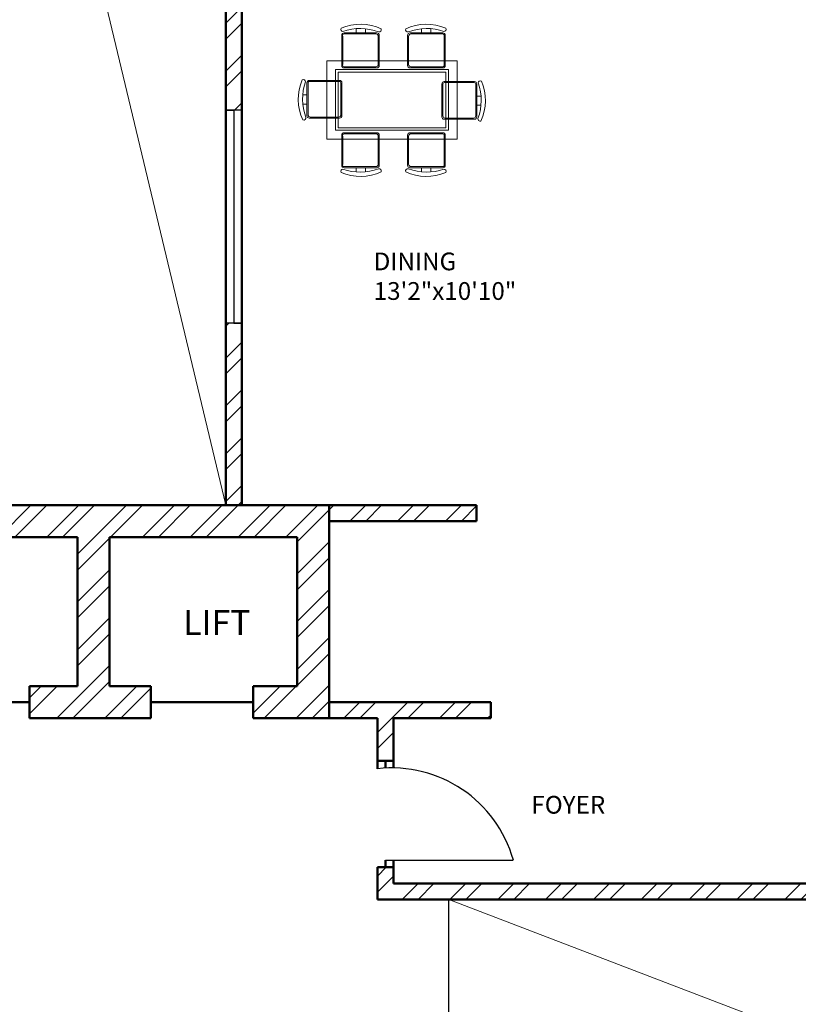
# Model space of a CAD drawing. Units: inches. Extents: x 1901 to 2863, y 888 to 2433.
# Tile 66 of 91: x 2381 to 2601, y 1732 to 2009. Entities that reach past the tile are written whole.
import ezdxf

# ---------------------------------------------------------------- set-up
doc = ezdxf.new("R2010")
doc.units = ezdxf.units.IN
for name, color, linetype, lineweight in [('A-ANNO-SYMB', 8, 'Continuous', 13), ('A-AREA-IDEN', 7, 'Continuous', 18), ('A-DOOR', 4, 'Continuous', 25), ('A-FLOR-HRAL', 41, 'Continuous', 25), ('A-FURN', 8, 'Continuous', 18), ('A-GLAZ', 3, 'Continuous', 25), ('A-WALL', 7, 'Continuous', 50), ('A-WALL-PATT', 8, 'Continuous', 13)]:
    doc.layers.add(name, color=color, linetype=linetype, lineweight=lineweight)
doc.styles.get("Standard").update_dxf_attribs({"font": 'arial.ttf'})

# ---------------------------------------------------------------- blocks, each defined once
blk = doc.blocks.new('WIN-60')
for p, q in [((0, 4.5), (0, 0)), ((60, 2.25), (60, 4.5)), ((60, 4.5), (60, 0)), ((0, 0), (0, 2.25)), ((0, 2.25), (60, 2.25))]:
    blk.add_line(p, q)

msp = doc.modelspace()

# ---------------------------------------------------------------- hatches: boundary and pattern name
at = {"layer": 'A-WALL-PATT'}
h = msp.add_hatch(dxfattribs=at)
h.set_pattern_fill('ANSI32', color=256)
h.paths.add_polyline_path([(2192.5, 2274.13), (2141.26, 2274.13), (2141.26, 2269.63), (2192.5, 2269.63)])
h.paths.add_polyline_path([(2259.93, 2274.13), (2216.5, 2274.13), (2216.5, 2269.63), (2255.43, 2269.63), (2255.43, 2214.63), (2250.81, 2214.63), (2250.81, 2210.13), (2259.93, 2210.13), (2259.93, 2215.13), (2271.76, 2215.13), (2271.76, 2217.38), (2271.76, 2219.63), (2259.93, 2219.63)])
h.paths.add_polyline_path([(2171.43, 2269.63), (2166.93, 2269.63), (2166.93, 2219.63), (2121.24, 2219.63), (2121.24, 2215.13), (2166.93, 2215.13), (2166.93, 2083.13), (2161.81, 2083.13), (2161.81, 2078.63), (2171.43, 2078.63), (2177, 2078.63), (2177, 2080.88), (2177, 2083.13), (2171.43, 2083.13), (2171.43, 2210.13), (2230.91, 2210.13), (2230.91, 2212.38), (2230.91, 2214.63), (2171.43, 2214.63)])
h.paths.add_polyline_path([(2117.26, 2274.13), (2089.43, 2274.13), (2089.43, 2219.63), (2081.14, 2219.63), (2081.14, 2215.13), (2089.43, 2215.13), (2098, 2215.13), (2098, 2217.38), (2098, 2219.63), (2093.93, 2219.63), (2093.93, 2269.63), (2117.26, 2269.63), (2117.26, 2271.88)])
h.paths.add_polyline_path([(2343.43, 2219.63), (2329.29, 2219.63), (2329.29, 2215.13), (2338.93, 2215.13), (2338.93, 2184.74), (2343.43, 2184.74)])
h.paths.add_polyline_path([(2338.93, 2083.13), (2329.29, 2083.13), (2208.97, 2083.13), (2208.97, 2078.63), (2338.93, 2078.63)])
h.paths.add_polyline_path([(2343.43, 2136.74), (2338.93, 2136.74), (2338.93, 1872.63), (2343.43, 1872.63)])
h.paths.add_polyline_path([(2343.43, 1863.63), (2397.68, 1863.63), (2397.68, 1821.63), (2384.14, 1821.63), (2384.14, 1812.63), (2418.33, 1812.63), (2418.33, 1817.13), (2418.33, 1821.63), (2406.68, 1821.63), (2406.68, 1863.63), (2459.5, 1863.63), (2459.5, 1821.63), (2447.14, 1821.63), (2447.14, 1812.63), (2459.5, 1812.63), (2468.5, 1812.63), (2468.5, 1872.63), (2394.43, 1872.63), (2334.43, 1872.63), (2334.43, 1812.63), (2343.43, 1812.63), (2353.25, 1812.63), (2353.25, 1821.63), (2343.43, 1821.63)])
h.paths.add_polyline_path([(2510.01, 1872.63), (2468.5, 1872.63), (2468.5, 1868.13), (2510.01, 1868.13)])
h.paths.add_polyline_path([(2514.01, 1817.13), (2468.5, 1817.13), (2468.5, 1812.63), (2482.11, 1812.63), (2482.11, 1800.61), (2486.61, 1800.61), (2486.61, 1812.63), (2514.01, 1812.63)])
h.paths.add_polyline_path([(2299.25, 1814.88), (2299.25, 1817.13), (2295.93, 1817.13), (2295.93, 1854.17), (2293.68, 1854.17), (2291.43, 1854.17), (2291.43, 1817.13), (2266.11, 1817.13), (2266.11, 1812.63), (2299.25, 1812.63)])
h.paths.add_polyline_path([(2218.11, 1817.13), (2206.46, 1817.13), (2171.43, 1817.13), (2171.43, 1949.13), (2190.1, 1949.13), (2190.1, 1953.63), (2163.47, 1953.63), (2163.47, 1949.13), (2166.93, 1949.13), (2166.93, 1817.13), (2114.3, 1817.13), (2114.3, 1812.63), (2218.11, 1812.63)])
h.paths.add_polyline_path([(2029.43, 1970.92), (2024.93, 1970.92), (2024.93, 1912.72), (2029.43, 1912.72)])
h.paths.add_polyline_path([(2132.3, 1953.63), (2113.93, 1953.63), (2113.93, 1975.89), (2111.68, 1975.89), (2109.43, 1975.89), (2109.43, 1953.63), (2029.43, 1953.63), (2029.43, 1949.13), (2132.3, 1949.13)])
h.paths.add_polyline_path([(2029.43, 1853.61), (2029.31, 1853.61), (2029.31, 1853.61), (2029.43, 1853.61), (2029.43, 1864.72), (2024.93, 1864.72), (2024.93, 1812.63), (2066.3, 1812.63), (2066.3, 1814.88), (2066.3, 1817.13), (2029.43, 1817.13)])
h.paths.add_polyline_path([(2122.93, 2010.09), (2120.68, 2010.09), (2118.43, 2010.09), (2118.43, 2006.13), (2029.43, 2006.13), (2029.43, 2001.63), (2109.43, 2001.63), (2109.43, 1998.04), (2113.93, 1998.04), (2113.93, 2001.63), (2122.93, 2001.63)])
h.paths.add_polyline_path([(2029.43, 2031.38), (2024.93, 2031.38), (2024.93, 1994.92), (2027.18, 1994.92), (2029.43, 1994.92)])
h.paths.add_polyline_path([(2029.43, 2136.74), (2024.93, 2136.74), (2024.93, 2067.38), (2027.18, 2067.38), (2029.43, 2067.38)])
h.paths.add_polyline_path([(2125.62, 2083.13), (2029.43, 2083.13), (2029.43, 2078.63), (2118.43, 2078.63), (2118.43, 2030.71), (2122.93, 2030.71), (2122.93, 2078.63), (2125.62, 2078.63)])
h.paths.add_polyline_path([(2029.43, 2215.13), (2040.47, 2215.13), (2040.47, 2217.38), (2040.47, 2219.63), (2024.93, 2219.63), (2024.93, 2184.74), (2029.43, 2184.74), (2029.43, 2187.78)])
h.paths.add_polyline_path([(2686.43, 2274.13), (2659.28, 2274.13), (2659.28, 2269.63), (2681.93, 2269.63), (2681.93, 2219.63), (2676.82, 2219.63), (2676.82, 2215.13), (2681.93, 2215.13), (2697.01, 2215.13), (2697.01, 2217.38), (2697.01, 2219.63), (2686.43, 2219.63)])
h.paths.add_polyline_path([(2609.93, 2269.63), (2635.28, 2269.63), (2635.28, 2274.13), (2571.43, 2274.13), (2571.43, 2269.63), (2605.43, 2269.63), (2605.43, 2214.63), (2549.1, 2214.63), (2549.1, 2210.13), (2605.43, 2210.13), (2605.43, 2083.13), (2601.01, 2083.13), (2601.01, 2080.88), (2601.01, 2078.63), (2609.93, 2078.63), (2616.16, 2078.63), (2616.16, 2080.88), (2616.16, 2083.13), (2609.93, 2083.13), (2609.93, 2215.13), (2651.46, 2215.13), (2651.46, 2217.38), (2651.46, 2219.63), (2609.93, 2219.63)])
h.paths.add_polyline_path([(2521.43, 2269.63), (2547.43, 2269.63), (2547.43, 2271.88), (2547.43, 2274.13), (2516.93, 2274.13), (2516.93, 2219.63), (2506.41, 2219.63), (2506.41, 2215.13), (2516.93, 2215.13), (2516.93, 2210.13), (2525.4, 2210.13), (2525.4, 2212.38), (2525.4, 2214.63), (2521.43, 2214.63)])
h.paths.add_polyline_path([(2456.01, 2219.63), (2439.43, 2219.63), (2439.43, 2187.89), (2443.93, 2187.89), (2443.93, 2215.13), (2456.01, 2215.13)])
h.paths.add_polyline_path([(2752.93, 2219.63), (2739.48, 2219.63), (2739.48, 2215.13), (2748.43, 2215.13), (2748.43, 2187.89), (2752.93, 2187.89)])
h.paths.add_polyline_path([(2752.93, 2139.89), (2748.43, 2139.89), (2748.43, 2083.13), (2648.42, 2083.13), (2648.42, 2078.63), (2654.93, 2078.63), (2654.93, 2039.44), (2659.43, 2039.44), (2659.43, 2078.63), (2748.43, 2078.63), (2748.43, 2063.43), (2752.93, 2063.43)])
h.paths.add_polyline_path([(2752.93, 2010.63), (2659.43, 2010.63), (2659.43, 2015.65), (2654.93, 2015.65), (2654.93, 2010.63), (2605.43, 2010.63), (2605.43, 1920.97), (2609.93, 1920.97), (2609.93, 2006.13), (2748.43, 2006.13), (2748.43, 1982.47), (2752.93, 1982.47)])
h.paths.add_polyline_path([(2752.93, 2027.43), (2748.43, 2027.43), (2748.43, 2010.63), (2752.93, 2010.63)])
h.paths.add_polyline_path([(2748.43, 1886.13), (2609.93, 1886.13), (2609.93, 1889.72), (2605.43, 1889.72), (2605.43, 1861.26), (2609.93, 1861.26), (2609.93, 1881.63), (2748.43, 1881.63)])
h.paths.add_polyline_path([(2456.86, 2228.83), (2498.4, 2228.83), (2498.4, 2247.49), (2456.86, 2247.49)], flags=9)
h.paths.add_polyline_path([(2038.6, 2237.42), (2080.17, 2237.42), (2080.17, 2256.08), (2038.6, 2256.08)], flags=9)
h.paths.add_polyline_path([(2292.01, 1062.39), (2539.93, 1062.39), (2539.93, 1099.49), (2292.01, 1099.49)], flags=9)
h.paths.add_polyline_path([(2424.91, 1832.25), (2448.51, 1832.25), (2448.51, 1846.68), (2424.91, 1846.68)], flags=25)
h.paths.add_polyline_path([(2359.08, 1832.25), (2382.68, 1832.25), (2382.68, 1846.68), (2359.08, 1846.68)], flags=25)
h.paths.add_polyline_path([(2352.9, 1684.8), (2367.54, 1684.8), (2367.54, 1697.17), (2352.9, 1697.17)], flags=9)
h.paths.add_polyline_path([(2079.29, 1755.83), (2169.02, 1755.83), (2169.02, 1774.37), (2079.29, 1774.37)], flags=9)
h.paths.add_polyline_path([(2404.09, 1373.86), (2404.09, 1463.59), (2385.54, 1463.59), (2385.54, 1373.86)], flags=9)
h.paths.add_polyline_path([(2268.09, 2236.37), (2309.64, 2236.37), (2309.64, 2255.03), (2268.09, 2255.03)], flags=9)
h.paths.add_polyline_path([(2575.96, 1700.95), (2665.7, 1700.95), (2665.7, 1719.5), (2575.96, 1719.5)], flags=9)
h.paths.add_polyline_path([(2302.96, 1878.47), (2329.52, 1878.47), (2329.52, 1888.78), (2302.96, 1888.78)], flags=9)
h.paths.add_polyline_path([(2097.42, 2240.58), (2126.57, 2240.58), (2126.57, 2259.23), (2097.42, 2259.23)], flags=9)
h.paths.add_polyline_path([(2208.72, 2246.12), (2237.88, 2246.12), (2237.88, 2264.78), (2208.72, 2264.78)], flags=9)
h.paths.add_polyline_path([(2038.15, 1925.96), (2076.99, 1925.96), (2076.99, 1944.62), (2038.15, 1944.62)], flags=9)
h.paths.add_polyline_path([(2239.14, 1926.67), (2288.46, 1926.67), (2288.46, 1945.33), (2239.14, 1945.33)], flags=9)
h.paths.add_polyline_path([(2175.43, 2007.33), (2212.36, 2007.33), (2212.36, 2025.99), (2175.43, 2025.99)], flags=9)
h.paths.add_polyline_path([(2225.03, 2091.79), (2263.87, 2091.79), (2263.87, 2110.45), (2225.03, 2110.45)], flags=9)
h.paths.add_polyline_path([(2035.4, 2098.48), (2074.24, 2098.48), (2074.24, 2117.14), (2035.4, 2117.14)], flags=9)
h.paths.add_polyline_path([(2050.1, 2029.21), (2083.26, 2029.21), (2083.26, 2047.87), (2050.1, 2047.87)], flags=9)
h.paths.add_polyline_path([(2069.68, 1956.72), (2098.83, 1956.72), (2098.83, 1975.38), (2069.68, 1975.38)], flags=25)
h.paths.add_polyline_path([(2328.62, 1753.34), (2361.66, 1753.34), (2361.66, 1771.99), (2328.62, 1771.99)], flags=9)
h.paths.add_polyline_path([(2395.16, 2060.89), (2395.16, 2140.65), (2378.68, 2140.65), (2378.68, 2060.89)], flags=9)
h.paths.add_polyline_path([(2463.73, 2059.02), (2492.89, 2059.02), (2492.89, 2077.68), (2463.73, 2077.68)], flags=9)
h.paths.add_polyline_path([(2458.03, 2181.54), (2496.87, 2181.54), (2496.87, 2200.19), (2458.03, 2200.19)], flags=9)
h.paths.add_polyline_path([(2527.58, 2243.07), (2556.73, 2243.07), (2556.73, 2261.73), (2527.58, 2261.73)], flags=9)
h.paths.add_polyline_path([(2694.46, 2232.77), (2736.03, 2232.77), (2736.03, 2251.42), (2694.46, 2251.42)], flags=9)
h.paths.add_polyline_path([(2637.82, 2249.22), (2666.98, 2249.22), (2666.98, 2267.88), (2637.82, 2267.88)], flags=9)
h.paths.add_polyline_path([(2623.69, 2183.54), (2662.53, 2183.54), (2662.53, 2202.2), (2623.69, 2202.2)], flags=9)
h.paths.add_polyline_path([(2691.97, 2021.5), (2725.12, 2021.5), (2725.12, 2040.16), (2691.97, 2040.16)], flags=9)
h.paths.add_polyline_path([(2621.04, 1975.91), (2662.34, 1975.91), (2662.34, 1994.57), (2621.04, 1994.57)], flags=25)
h.paths.add_polyline_path([(2479.03, 1927.62), (2519.84, 1927.62), (2519.84, 1946.28), (2479.03, 1946.28)], flags=9)
h.paths.add_polyline_path([(2670.94, 1849.08), (2716.01, 1849.08), (2716.01, 1867.73), (2670.94, 1867.73)], flags=9)
h.paths.add_polyline_path([(2523.61, 1782.96), (2550.17, 1782.96), (2550.17, 1793.26), (2523.61, 1793.26)], flags=9)
h.paths.add_polyline_path([(2450.84, 1207.33), (2492.39, 1207.33), (2492.39, 1225.99), (2450.84, 1225.99)], flags=9)
h.paths.add_polyline_path([(2527.75, 1203.84), (2556.91, 1203.84), (2556.91, 1222.5), (2527.75, 1222.5)], flags=9)
h.paths.add_polyline_path([(2639.11, 1207.2), (2668.27, 1207.2), (2668.27, 1225.86), (2639.11, 1225.86)], flags=9)
h.paths.add_polyline_path([(2692.59, 1218.97), (2734.17, 1218.97), (2734.17, 1237.62), (2692.59, 1237.62)], flags=9)
h.paths.add_polyline_path([(2669.27, 1366.33), (2708.11, 1366.33), (2708.11, 1384.99), (2669.27, 1384.99)], flags=9)
h.paths.add_polyline_path([(2463.31, 1358.03), (2502.15, 1358.03), (2502.15, 1376.69), (2463.31, 1376.69)], flags=9)
h.paths.add_polyline_path([(2494.72, 1449.96), (2531.65, 1449.96), (2531.65, 1468.62), (2494.72, 1468.62)], flags=9)
h.paths.add_polyline_path([(2675.57, 1422.16), (2708.72, 1422.16), (2708.72, 1440.81), (2675.57, 1440.81)], flags=9)
h.paths.add_polyline_path([(2685.63, 1493.89), (2714.79, 1493.89), (2714.79, 1512.55), (2685.63, 1512.55)], flags=9)
h.paths.add_polyline_path([(2686.8, 1529.91), (2725.65, 1529.91), (2725.65, 1548.57), (2686.8, 1548.57)], flags=9)
h.paths.add_polyline_path([(2503.65, 1537.99), (2552.97, 1537.99), (2552.97, 1556.65), (2503.65, 1556.65)], flags=9)
h.paths.add_polyline_path([(2291.71, 1643.5), (2318.28, 1643.5), (2318.28, 1653.81), (2291.71, 1653.81)], flags=9)
h.paths.add_polyline_path([(2450.63, 1610.52), (2477.19, 1610.52), (2477.19, 1620.82), (2450.63, 1620.82)], flags=9)
h.paths.add_polyline_path([(2359.99, 1551.81), (2422.25, 1551.81), (2422.25, 1562.12), (2359.99, 1562.12)], flags=9)
h.paths.add_polyline_path([(2280.11, 1249.01), (2321.65, 1249.01), (2321.65, 1267.66), (2280.11, 1267.66)], flags=9)
h.paths.add_polyline_path([(2164.06, 1274.23), (2193.22, 1274.23), (2193.22, 1292.89), (2164.06, 1292.89)], flags=9)
h.paths.add_polyline_path([(2118.21, 1277.69), (2151.25, 1277.69), (2151.25, 1296.35), (2118.21, 1296.35)], flags=9)
h.paths.add_polyline_path([(2031.95, 1268.53), (2073.52, 1268.53), (2073.52, 1287.19), (2031.95, 1287.19)], flags=9)
h.paths.add_polyline_path([(2050.2, 1409.08), (2089.04, 1409.08), (2089.04, 1427.74), (2050.2, 1427.74)], flags=9)
h.paths.add_polyline_path([(2243.74, 1421.03), (2282.58, 1421.03), (2282.58, 1439.69), (2243.74, 1439.69)], flags=9)
h.paths.add_polyline_path([(2190.75, 1509.77), (2231.56, 1509.77), (2231.56, 1528.43), (2190.75, 1528.43)], flags=9)
h.paths.add_polyline_path([(2058.39, 1475.42), (2091.55, 1475.42), (2091.55, 1494.07), (2058.39, 1494.07)], flags=9)
h.paths.add_polyline_path([(2062.45, 1553.09), (2091.6, 1553.09), (2091.6, 1571.75), (2062.45, 1571.75)], flags=9)
h.paths.add_polyline_path([(2219.52, 1590.37), (2266.15, 1590.37), (2266.15, 1609.02), (2219.52, 1609.02)], flags=9)
h.paths.add_polyline_path([(2041.07, 1584.19), (2079.91, 1584.19), (2079.91, 1602.85), (2041.07, 1602.85)], flags=9)
h = msp.add_hatch(dxfattribs=at)
h.set_pattern_fill('ANSI32', color=256)
h.paths.add_polyline_path([(2443.93, 2139.89), (2439.43, 2139.89), (2439.43, 2069.35), (2441.68, 2069.35), (2443.93, 2069.35), (2443.93, 2078.63), (2521.93, 2078.63), (2521.93, 2075.07), (2524.18, 2075.07), (2526.43, 2075.07), (2526.43, 2078.63), (2571.75, 2078.63), (2571.75, 2080.88), (2571.75, 2083.13), (2443.93, 2083.13)])
h.paths.add_polyline_path([(2526.43, 2054.63), (2524.18, 2054.63), (2521.93, 2054.63), (2521.93, 2030.63), (2443.93, 2030.63), (2443.93, 2045.35), (2439.43, 2045.35), (2439.43, 1983.87), (2443.93, 1983.87), (2443.93, 2026.13), (2521.93, 2026.13), (2526.43, 2026.13)])
h.paths.add_polyline_path([(2443.93, 1923.87), (2439.43, 1923.87), (2439.43, 1872.63), (2443.93, 1872.63)])
h.paths.add_polyline_path([(2636.23, 1766.13), (2609.93, 1766.13), (2609.93, 1779.79), (2605.43, 1779.79), (2605.43, 1766.13), (2486.61, 1766.13), (2486.61, 1770.67), (2482.11, 1770.67), (2482.11, 1766.13), (2482.11, 1761.63), (2636.23, 1761.63), (2636.23, 1763.88)])
h.paths.add_polyline_path([(2519.54, 1663.38), (2519.54, 1665.63), (2494.93, 1665.63), (2481.83, 1665.63), (2481.83, 1663.38), (2481.83, 1661.13), (2490.43, 1661.13), (2490.43, 1640.16), (2494.93, 1640.16), (2494.93, 1661.13), (2519.54, 1661.13)])
h.paths.add_polyline_path([(2443.93, 1712.13), (2443.93, 1716.63), (2414.46, 1716.63), (2414.46, 1712.13), (2439.43, 1712.13), (2439.43, 1545.51), (2443.93, 1545.51), (2443.93, 1661.13), (2448.47, 1661.13), (2448.47, 1665.63), (2443.93, 1665.63)])
h.paths.add_polyline_path([(2343.43, 1712.13), (2365.52, 1712.13), (2365.52, 1714.38), (2365.52, 1716.63), (2333.87, 1716.63), (2333.87, 1714.38), (2333.87, 1712.13), (2338.93, 1712.13), (2338.93, 1575.63), (2338.93, 1545.51), (2343.43, 1545.51), (2343.43, 1547.51), (2343.43, 1580.13)])
h.paths.add_polyline_path([(2752.93, 1665.63), (2579.54, 1665.63), (2579.54, 1661.13), (2615.93, 1661.13), (2615.93, 1529.13), (2598.93, 1529.13), (2598.93, 1524.63), (2623.13, 1524.63), (2623.13, 1526.88), (2623.13, 1529.13), (2620.43, 1529.13), (2620.43, 1661.13), (2748.43, 1661.13), (2748.43, 1633.5), (2752.93, 1633.5)])
h.paths.add_polyline_path([(2752.93, 1419.93), (2748.43, 1419.93), (2748.43, 1400.13), (2659.43, 1400.13), (2659.43, 1444.33), (2657.18, 1444.33), (2654.93, 1444.33), (2654.93, 1400.13), (2643.65, 1400.13), (2643.65, 1395.63), (2748.43, 1395.63), (2748.43, 1364.04), (2752.93, 1364.04)])
h.paths.add_polyline_path([(2752.93, 1492.88), (2748.43, 1492.88), (2748.43, 1476.63), (2667.43, 1476.63), (2667.43, 1479.71), (2665.18, 1479.71), (2662.93, 1479.71), (2662.93, 1476.63), (2654.93, 1476.63), (2654.93, 1469.54), (2659.43, 1469.54), (2659.43, 1472.13), (2748.43, 1472.13), (2748.43, 1455.93), (2752.93, 1455.93)])
h.paths.add_polyline_path([(2752.93, 1304.04), (2748.43, 1304.04), (2748.43, 1263.63), (2738.66, 1263.63), (2738.66, 1259.13), (2752.93, 1259.13)])
h.paths.add_polyline_path([(2685.93, 1259.13), (2695.49, 1259.13), (2695.49, 1261.38), (2695.49, 1263.63), (2677.84, 1263.63), (2677.84, 1261.38), (2677.84, 1259.13), (2681.43, 1259.13), (2681.43, 1203.63), (2653.28, 1203.63), (2653.28, 1199.13), (2685.93, 1199.13), (2685.93, 1203.63)])
h.paths.add_polyline_path([(2609.43, 1395.63), (2611.85, 1395.63), (2611.85, 1400.13), (2598.89, 1400.13), (2598.89, 1397.88), (2598.89, 1395.63), (2604.93, 1395.63), (2604.93, 1268.13), (2554.73, 1268.13), (2554.73, 1265.88), (2554.73, 1263.63), (2604.93, 1263.63), (2604.93, 1203.63), (2571.31, 1203.63), (2571.31, 1199.13), (2604.93, 1199.13), (2629.28, 1199.13), (2629.28, 1201.38), (2629.28, 1203.63), (2609.43, 1203.63), (2609.43, 1258.63), (2609.43, 1259.13), (2654.8, 1259.13), (2654.8, 1263.63), (2609.43, 1263.63)])
h.paths.add_polyline_path([(2443.93, 1304.04), (2439.43, 1304.04), (2439.43, 1259.13), (2443.93, 1259.13), (2456.16, 1259.13), (2456.16, 1261.38), (2456.16, 1263.63), (2443.93, 1263.63)])
h.paths.add_polyline_path([(2525.43, 1263.63), (2531.78, 1263.63), (2531.78, 1268.13), (2520.93, 1268.13), (2520.93, 1263.63), (2511.41, 1263.63), (2511.41, 1259.13), (2520.93, 1259.13), (2520.93, 1199.13), (2547.31, 1199.13), (2547.31, 1201.38), (2547.31, 1203.63), (2525.43, 1203.63)])
h.paths.add_polyline_path([(2443.93, 1434.84), (2439.43, 1434.84), (2439.43, 1364.04), (2441.68, 1364.04), (2443.93, 1364.04)])
h.paths.add_polyline_path([(2567.13, 1400.13), (2443.93, 1400.13), (2443.93, 1395.63), (2567.13, 1395.63)])
h.paths.add_polyline_path([(2443.93, 1545.51), (2439.43, 1545.51), (2439.43, 1494.84), (2443.93, 1494.84)])
h.paths.add_polyline_path([(2494.93, 1553.35), (2492.68, 1553.35), (2490.43, 1553.35), (2490.43, 1524.63), (2494.93, 1524.63), (2525.94, 1524.63), (2525.94, 1526.88), (2525.94, 1529.13), (2494.93, 1529.13)])
h.paths.add_polyline_path([(2752.93, 1573.5), (2748.43, 1573.5), (2748.43, 1529.13), (2657.76, 1529.13), (2657.76, 1524.63), (2662.93, 1524.63), (2662.93, 1498.63), (2667.43, 1498.63), (2667.43, 1524.63), (2748.43, 1524.63), (2748.43, 1516.88), (2752.93, 1516.88)])
h.paths.add_polyline_path([(2038.6, 2237.42), (2080.17, 2237.42), (2080.17, 2256.08), (2038.6, 2256.08)], flags=9)
h.paths.add_polyline_path([(2292.01, 1062.39), (2539.93, 1062.39), (2539.93, 1099.49), (2292.01, 1099.49)], flags=9)
h.paths.add_polyline_path([(2424.91, 1832.25), (2448.51, 1832.25), (2448.51, 1846.68), (2424.91, 1846.68)], flags=9)
h.paths.add_polyline_path([(2359.08, 1832.25), (2382.68, 1832.25), (2382.68, 1846.68), (2359.08, 1846.68)], flags=9)
h.paths.add_polyline_path([(2352.9, 1684.8), (2367.54, 1684.8), (2367.54, 1697.17), (2352.9, 1697.17)], flags=9)
h.paths.add_polyline_path([(2079.29, 1755.83), (2169.02, 1755.83), (2169.02, 1774.37), (2079.29, 1774.37)], flags=9)
h.paths.add_polyline_path([(2404.09, 1373.86), (2404.09, 1463.59), (2385.54, 1463.59), (2385.54, 1373.86)], flags=9)
h.paths.add_polyline_path([(2268.09, 2236.37), (2309.64, 2236.37), (2309.64, 2255.03), (2268.09, 2255.03)], flags=9)
h.paths.add_polyline_path([(2575.96, 1700.95), (2665.7, 1700.95), (2665.7, 1719.5), (2575.96, 1719.5)], flags=9)
h.paths.add_polyline_path([(2302.96, 1878.47), (2329.52, 1878.47), (2329.52, 1888.78), (2302.96, 1888.78)], flags=9)
h.paths.add_polyline_path([(2097.42, 2240.58), (2126.57, 2240.58), (2126.57, 2259.23), (2097.42, 2259.23)], flags=9)
h.paths.add_polyline_path([(2208.72, 2246.12), (2237.88, 2246.12), (2237.88, 2264.78), (2208.72, 2264.78)], flags=9)
h.paths.add_polyline_path([(2038.15, 1925.96), (2076.99, 1925.96), (2076.99, 1944.62), (2038.15, 1944.62)], flags=9)
h.paths.add_polyline_path([(2239.14, 1926.67), (2288.46, 1926.67), (2288.46, 1945.33), (2239.14, 1945.33)], flags=9)
h.paths.add_polyline_path([(2175.43, 2007.33), (2212.36, 2007.33), (2212.36, 2025.99), (2175.43, 2025.99)], flags=9)
h.paths.add_polyline_path([(2225.03, 2091.79), (2263.87, 2091.79), (2263.87, 2110.45), (2225.03, 2110.45)], flags=9)
h.paths.add_polyline_path([(2035.4, 2098.48), (2074.24, 2098.48), (2074.24, 2117.14), (2035.4, 2117.14)], flags=9)
h.paths.add_polyline_path([(2050.1, 2029.21), (2083.26, 2029.21), (2083.26, 2047.87), (2050.1, 2047.87)], flags=9)
h.paths.add_polyline_path([(2069.68, 1956.72), (2098.83, 1956.72), (2098.83, 1975.38), (2069.68, 1975.38)], flags=9)
h.paths.add_polyline_path([(2328.62, 1753.34), (2361.66, 1753.34), (2361.66, 1771.99), (2328.62, 1771.99)], flags=9)
h.paths.add_polyline_path([(2395.16, 2060.89), (2395.16, 2140.65), (2378.68, 2140.65), (2378.68, 2060.89)], flags=9)
h.paths.add_polyline_path([(2463.73, 2059.02), (2492.89, 2059.02), (2492.89, 2077.68), (2463.73, 2077.68)], flags=9)
h.paths.add_polyline_path([(2458.03, 2181.54), (2496.87, 2181.54), (2496.87, 2200.19), (2458.03, 2200.19)], flags=9)
h.paths.add_polyline_path([(2456.86, 2228.83), (2498.4, 2228.83), (2498.4, 2247.49), (2456.86, 2247.49)], flags=9)
h.paths.add_polyline_path([(2527.58, 2243.07), (2556.73, 2243.07), (2556.73, 2261.73), (2527.58, 2261.73)], flags=9)
h.paths.add_polyline_path([(2694.46, 2232.77), (2736.03, 2232.77), (2736.03, 2251.42), (2694.46, 2251.42)], flags=9)
h.paths.add_polyline_path([(2637.82, 2249.22), (2666.98, 2249.22), (2666.98, 2267.88), (2637.82, 2267.88)], flags=9)
h.paths.add_polyline_path([(2623.69, 2183.54), (2662.53, 2183.54), (2662.53, 2202.2), (2623.69, 2202.2)], flags=9)
h.paths.add_polyline_path([(2691.97, 2021.5), (2725.12, 2021.5), (2725.12, 2040.16), (2691.97, 2040.16)], flags=9)
h.paths.add_polyline_path([(2621.04, 1975.91), (2662.34, 1975.91), (2662.34, 1994.57), (2621.04, 1994.57)], flags=9)
h.paths.add_polyline_path([(2479.03, 1927.62), (2519.84, 1927.62), (2519.84, 1946.28), (2479.03, 1946.28)], flags=9)
h.paths.add_polyline_path([(2670.94, 1849.08), (2716.01, 1849.08), (2716.01, 1867.73), (2670.94, 1867.73)], flags=9)
h.paths.add_polyline_path([(2523.61, 1782.96), (2550.17, 1782.96), (2550.17, 1793.26), (2523.61, 1793.26)], flags=9)
h.paths.add_polyline_path([(2450.84, 1207.33), (2492.39, 1207.33), (2492.39, 1225.99), (2450.84, 1225.99)], flags=9)
h.paths.add_polyline_path([(2527.75, 1203.84), (2556.91, 1203.84), (2556.91, 1222.5), (2527.75, 1222.5)], flags=9)
h.paths.add_polyline_path([(2639.11, 1207.2), (2668.27, 1207.2), (2668.27, 1225.86), (2639.11, 1225.86)], flags=9)
h.paths.add_polyline_path([(2692.59, 1218.97), (2734.17, 1218.97), (2734.17, 1237.62), (2692.59, 1237.62)], flags=9)
h.paths.add_polyline_path([(2669.27, 1366.33), (2708.11, 1366.33), (2708.11, 1384.99), (2669.27, 1384.99)], flags=25)
h.paths.add_polyline_path([(2463.31, 1358.03), (2502.15, 1358.03), (2502.15, 1376.69), (2463.31, 1376.69)], flags=9)
h.paths.add_polyline_path([(2494.72, 1449.96), (2531.65, 1449.96), (2531.65, 1468.62), (2494.72, 1468.62)], flags=9)
h.paths.add_polyline_path([(2675.57, 1422.16), (2708.72, 1422.16), (2708.72, 1440.81), (2675.57, 1440.81)], flags=25)
h.paths.add_polyline_path([(2685.63, 1493.89), (2714.79, 1493.89), (2714.79, 1512.55), (2685.63, 1512.55)], flags=9)
h.paths.add_polyline_path([(2686.8, 1529.91), (2725.65, 1529.91), (2725.65, 1548.57), (2686.8, 1548.57)], flags=25)
h.paths.add_polyline_path([(2503.65, 1537.99), (2552.97, 1537.99), (2552.97, 1556.65), (2503.65, 1556.65)], flags=9)
h.paths.add_polyline_path([(2291.71, 1643.5), (2318.28, 1643.5), (2318.28, 1653.81), (2291.71, 1653.81)], flags=9)
h.paths.add_polyline_path([(2450.63, 1610.52), (2477.19, 1610.52), (2477.19, 1620.82), (2450.63, 1620.82)], flags=9)
h.paths.add_polyline_path([(2359.99, 1551.81), (2422.25, 1551.81), (2422.25, 1562.12), (2359.99, 1562.12)], flags=9)
h.paths.add_polyline_path([(2280.11, 1249.01), (2321.65, 1249.01), (2321.65, 1267.66), (2280.11, 1267.66)], flags=9)
h.paths.add_polyline_path([(2164.06, 1274.23), (2193.22, 1274.23), (2193.22, 1292.89), (2164.06, 1292.89)], flags=9)
h.paths.add_polyline_path([(2118.21, 1277.69), (2151.25, 1277.69), (2151.25, 1296.35), (2118.21, 1296.35)], flags=9)
h.paths.add_polyline_path([(2031.95, 1268.53), (2073.52, 1268.53), (2073.52, 1287.19), (2031.95, 1287.19)], flags=9)
h.paths.add_polyline_path([(2050.2, 1409.08), (2089.04, 1409.08), (2089.04, 1427.74), (2050.2, 1427.74)], flags=9)
h.paths.add_polyline_path([(2243.74, 1421.03), (2282.58, 1421.03), (2282.58, 1439.69), (2243.74, 1439.69)], flags=9)
h.paths.add_polyline_path([(2190.75, 1509.77), (2231.56, 1509.77), (2231.56, 1528.43), (2190.75, 1528.43)], flags=9)
h.paths.add_polyline_path([(2058.39, 1475.42), (2091.55, 1475.42), (2091.55, 1494.07), (2058.39, 1494.07)], flags=9)
h.paths.add_polyline_path([(2062.45, 1553.09), (2091.6, 1553.09), (2091.6, 1571.75), (2062.45, 1571.75)], flags=9)
h.paths.add_polyline_path([(2219.52, 1590.37), (2266.15, 1590.37), (2266.15, 1609.02), (2219.52, 1609.02)], flags=9)
h.paths.add_polyline_path([(2041.07, 1584.19), (2079.91, 1584.19), (2079.91, 1602.85), (2041.07, 1602.85)], flags=9)

# ---------------------------------------------------------------- linework, layer by layer
at = {"layer": 'A-ANNO-SYMB'}
for p, q in [((2343.43, 2274.13), (2439.43, 1872.63)), ((2502.24, 1761.63), (2752.93, 1665.63))]:
    msp.add_line(p, q, dxfattribs=at)
at = {"layer": 'A-DOOR'}
msp.add_line((2484.36, 1772.67), (2520.36, 1772.67), dxfattribs=at)
msp.add_arc((2486.08, 1763.03), 35.62, 15.7074, 96.3857, dxfattribs=at)
at = {"layer": 'A-FLOR-HRAL'}
msp.add_line((2502.24, 1665.63), (2502.24, 1761.63), dxfattribs=at)
at = {"layer": 'A-FURN'}
for points in [[(2472.39, 2006.04, -0.175809), (2482.4, 2005.96, 0.578392), (2483.16, 2006.79, 0.214524), (2471.86, 2006.94, 0.552014), (2472.39, 2006.04, -0.065079)], [(2472.39, 2006.04, -0.175809), (2482.4, 2005.96, 0.578392), (2483.16, 2006.79, 0.214524), (2471.86, 2006.94, 0.552014), (2472.39, 2006.04, -0.065079)], [(2490.82, 2005.96, -0.578392), (2490.06, 2006.79, -0.214524), (2501.35, 2006.94, -0.552014), (2500.82, 2006.04, 0.175809), (2490.82, 2005.96)], [(2490.82, 2005.96, -0.578392), (2490.06, 2006.79, -0.214524), (2501.35, 2006.94, -0.552014), (2500.82, 2006.04, 0.175809), (2490.82, 2005.96)], [(2481.97, 2005.63), (2472.69, 2005.63, 0.414214), (2472.04, 2004.98), (2472.04, 1996.45, 0.414214), (2472.69, 1995.8), (2481.97, 1995.8, 0.414214), (2482.62, 1996.45), (2482.62, 2004.98, 0.414214), (2481.97, 2005.63)], [(2481.97, 2005.63), (2472.69, 2005.63, 0.414214), (2472.04, 2004.98), (2472.04, 1996.44, 0.414214), (2472.69, 1995.79), (2481.97, 1995.79, 0.414214), (2482.62, 1996.44), (2482.62, 2004.98, 0.414214), (2481.97, 2005.63)], [(2478.71, 2005.63), (2478.71, 2006.81, -0.064759)], [(2478.71, 2005.63), (2478.71, 2006.81, -0.064759)], [(2500.53, 2005.63, -0.414214), (2501.18, 2004.98), (2501.18, 1996.45, -0.414214), (2500.53, 1995.8), (2491.24, 1995.8, -0.414214), (2490.59, 1996.45), (2490.59, 2004.98, -0.414214), (2491.24, 2005.63), (2500.53, 2005.63)], [(2500.53, 2005.63, -0.414214), (2501.18, 2004.98), (2501.18, 1996.44, -0.414214), (2500.53, 1995.79), (2491.24, 1995.79, -0.414214), (2490.59, 1996.44), (2490.59, 2004.98, -0.414214), (2491.24, 2005.63), (2500.53, 2005.63)], [(2494.51, 2005.63), (2494.51, 2006.81, 0.064759)], [(2494.51, 2005.63), (2494.51, 2006.81, 0.064759)], [(2461.93, 1981.88, -0.578392), (2461.1, 1981.12, -0.214524), (2460.94, 1992.41, -0.552014), (2461.85, 1991.88, 0.175809), (2461.93, 1981.88)], [(2461.93, 1981.88, -0.578392), (2461.1, 1981.12, -0.214524), (2460.94, 1992.41, -0.552014), (2461.85, 1991.88, 0.175809), (2461.93, 1981.88)], [(2462.25, 1991.59, -0.414214), (2462.9, 1992.24), (2471.44, 1992.24, -0.414214), (2472.09, 1991.59), (2472.09, 1982.3, -0.414214), (2471.44, 1981.65), (2462.9, 1981.65, -0.414214), (2462.25, 1982.3), (2462.25, 1991.59)], [(2462.25, 1991.59, -0.414214), (2462.9, 1992.24), (2471.44, 1992.24, -0.414214), (2472.09, 1991.59), (2472.09, 1982.3, -0.414214), (2471.44, 1981.65), (2462.9, 1981.65, -0.414214), (2462.25, 1982.3), (2462.25, 1991.59)], [(2510.08, 1991.27, 0.414214), (2509.43, 1991.92), (2500.89, 1991.92, 0.414214), (2500.24, 1991.27), (2500.24, 1981.98, 0.414214), (2500.89, 1981.33), (2509.43, 1981.33, 0.414214), (2510.08, 1981.98), (2510.08, 1991.27)], [(2510.08, 1991.27, 0.414214), (2509.43, 1991.92), (2500.89, 1991.92, 0.414214), (2500.24, 1991.27), (2500.24, 1981.98, 0.414214), (2500.89, 1981.33), (2509.43, 1981.33, 0.414214), (2510.08, 1981.98), (2510.08, 1991.27)], [(2510.48, 1991.56, -0.175809), (2510.4, 1981.56, 0.578392), (2511.24, 1980.8, 0.214524), (2511.39, 1992.09, 0.552014), (2510.48, 1991.56, -0.065079)], [(2510.48, 1991.56, -0.175809), (2510.4, 1981.56, 0.578392), (2511.24, 1980.8, 0.214524), (2511.39, 1992.09, 0.552014), (2510.48, 1991.56, -0.065079)], [(2462.25, 1985.56), (2461.08, 1985.56, 0.064759)], [(2462.25, 1985.56), (2461.08, 1985.56, 0.064759)], [(2510.08, 1985.25), (2511.25, 1985.25, -0.064759)], [(2510.08, 1985.25), (2511.25, 1985.25, -0.064759)], [(2481.97, 1967.68), (2472.69, 1967.68, -0.414214), (2472.04, 1968.32), (2472.04, 1976.86, -0.414214), (2472.69, 1977.51), (2481.97, 1977.51, -0.414214), (2482.62, 1976.86), (2482.62, 1968.32, -0.414214), (2481.97, 1967.68)], [(2481.97, 1967.67), (2472.69, 1967.67, -0.414214), (2472.04, 1968.32), (2472.04, 1976.86, -0.414214), (2472.69, 1977.51), (2481.97, 1977.51, -0.414214), (2482.62, 1976.86), (2482.62, 1968.32, -0.414214), (2481.97, 1967.67)], [(2500.53, 1967.68, 0.414214), (2501.18, 1968.32), (2501.18, 1976.86, 0.414214), (2500.53, 1977.51), (2491.24, 1977.51, 0.414214), (2490.59, 1976.86), (2490.59, 1968.32, 0.414214), (2491.24, 1967.68), (2500.53, 1967.68)], [(2500.53, 1967.67, 0.414214), (2501.18, 1968.32), (2501.18, 1976.86, 0.414214), (2500.53, 1977.51), (2491.24, 1977.51, 0.414214), (2490.59, 1976.86), (2490.59, 1968.32, 0.414214), (2491.24, 1967.67), (2500.53, 1967.67)], [(2482.4, 1967.35, -0.578392), (2483.16, 1966.52, -0.214524), (2471.86, 1966.36, -0.552014), (2472.39, 1967.27, 0.175809), (2482.4, 1967.35)], [(2482.4, 1967.35, -0.578392), (2483.16, 1966.52, -0.214524), (2471.86, 1966.36, -0.552014), (2472.39, 1967.27, 0.175809), (2482.4, 1967.35)], [(2478.71, 1967.68), (2478.71, 1966.5, 0.064759)], [(2478.71, 1967.67), (2478.71, 1966.5, 0.064759)], [(2500.82, 1967.27, -0.175809), (2490.82, 1967.35, 0.578392), (2490.06, 1966.52, 0.214524), (2501.35, 1966.36, 0.552014), (2500.82, 1967.27, -0.065079)], [(2500.82, 1967.27, -0.175809), (2490.82, 1967.35, 0.578392), (2490.06, 1966.52, 0.214524), (2501.35, 1966.36, 0.552014), (2500.82, 1967.27, -0.065079)], [(2494.51, 1967.68), (2494.51, 1966.5, -0.064759)], [(2494.51, 1967.67), (2494.51, 1966.5, -0.064759)]]:
    msp.add_lwpolyline(points, format="xyb", dxfattribs=at)
for points in [[(2472.69, 2005.34), (2481.68, 2005.34, -0.414214), (2482.33, 2004.69), (2482.33, 1996.74, -0.414214), (2481.68, 1996.09), (2472.69, 1996.09, -0.512069), (2472.33, 1996.74), (2472.33, 2004.69, -0.512069)], [(2472.69, 2005.34), (2481.68, 2005.34, -0.414214), (2482.33, 2004.69), (2482.33, 1996.74, -0.414214), (2481.68, 1996.09), (2472.69, 1996.09, -0.512069), (2472.33, 1996.74), (2472.33, 2004.69, -0.512069)], [(2500.53, 2005.34), (2491.54, 2005.34, 0.414214), (2490.89, 2004.69), (2490.89, 1996.74, 0.414214), (2491.54, 1996.09), (2500.53, 1996.09, 0.512069), (2500.89, 1996.74), (2500.89, 2004.69, 0.512069)], [(2500.53, 2005.34), (2491.54, 2005.34, 0.414214), (2490.89, 2004.69), (2490.89, 1996.74, 0.414214), (2491.54, 1996.09), (2500.53, 1996.09, 0.512069), (2500.89, 1996.74), (2500.89, 2004.69, 0.512069)], [(2462.55, 1991.59), (2462.55, 1982.6, 0.414214), (2463.2, 1981.95), (2471.15, 1981.95, 0.414214), (2471.8, 1982.6), (2471.8, 1991.59, 0.512069), (2471.15, 1991.95), (2463.2, 1991.95, 0.512069)], [(2462.55, 1991.59), (2462.55, 1982.6, 0.414214), (2463.2, 1981.95), (2471.15, 1981.95, 0.414214), (2471.8, 1982.6), (2471.8, 1991.59, 0.512069), (2471.15, 1991.95), (2463.2, 1991.95, 0.512069)], [(2509.78, 1991.27), (2509.78, 1982.28, -0.414214), (2509.14, 1981.63), (2501.18, 1981.63, -0.414214), (2500.53, 1982.28), (2500.53, 1991.27, -0.512069), (2501.18, 1991.63), (2509.14, 1991.63, -0.512069)], [(2509.78, 1991.27), (2509.78, 1982.28, -0.414214), (2509.14, 1981.63), (2501.18, 1981.63, -0.414214), (2500.53, 1982.28), (2500.53, 1991.27, -0.512069), (2501.18, 1991.63), (2509.14, 1991.63, -0.512069)], [(2472.69, 1967.97), (2481.68, 1967.97, 0.414214), (2482.33, 1968.62), (2482.33, 1976.57, 0.414214), (2481.68, 1977.22), (2472.69, 1977.22, 0.512069), (2472.33, 1976.57), (2472.33, 1968.62, 0.512069)], [(2472.69, 1967.97), (2481.68, 1967.97, 0.414214), (2482.33, 1968.62), (2482.33, 1976.57, 0.414214), (2481.68, 1977.22), (2472.69, 1977.22, 0.512069), (2472.33, 1976.57), (2472.33, 1968.62, 0.512069)], [(2500.53, 1967.97), (2491.54, 1967.97, -0.414214), (2490.89, 1968.62), (2490.89, 1976.57, -0.414214), (2491.54, 1977.22), (2500.53, 1977.22, -0.512069), (2500.89, 1976.57), (2500.89, 1968.62, -0.512069)], [(2500.53, 1967.97), (2491.54, 1967.97, -0.414214), (2490.89, 1968.62), (2490.89, 1976.57, -0.414214), (2491.54, 1977.22), (2500.53, 1977.22, -0.512069), (2500.89, 1976.57), (2500.89, 1968.62, -0.512069)]]:
    msp.add_lwpolyline(points, format="xyb", close=True, dxfattribs=at)
for points in [[(2476.11, 2006.83), (2476.11, 2005.63)], [(2476.11, 2006.83), (2476.11, 2005.63)], [(2497.11, 2006.83), (2497.11, 2005.63)], [(2497.11, 2006.83), (2497.11, 2005.63)], [(2461.06, 1988.16), (2462.25, 1988.16)], [(2461.06, 1988.16), (2462.25, 1988.16)], [(2511.27, 1987.85), (2510.08, 1987.85)], [(2511.27, 1987.85), (2510.08, 1987.85)], [(2476.11, 1966.48), (2476.11, 1967.68)], [(2476.11, 1966.48), (2476.11, 1967.67)], [(2497.11, 1966.48), (2497.11, 1967.68)], [(2497.11, 1966.48), (2497.11, 1967.67)]]:
    msp.add_lwpolyline(points, dxfattribs=at)
for points in [[(2467.85, 1997.79), (2504.58, 1997.79), (2504.58, 1975.75), (2467.85, 1975.75)], [(2467.85, 1997.79), (2504.58, 1997.79), (2504.58, 1975.75), (2467.85, 1975.75)], [(2470.3, 1995.34), (2502.13, 1995.34), (2502.13, 1978.2), (2470.3, 1978.2)], [(2470.3, 1995.34), (2502.13, 1995.34), (2502.13, 1978.2), (2470.3, 1978.2)], [(2471.03, 1994.61), (2501.4, 1994.61), (2501.4, 1978.94), (2471.03, 1978.94)], [(2471.03, 1994.61), (2501.4, 1994.61), (2501.4, 1978.94), (2471.03, 1978.94)]]:
    msp.add_lwpolyline(points, close=True, dxfattribs=at)
at = {"layer": 'A-WALL'}
for p, q in [((2439.43, 2219.63), (2439.43, 1872.63)), ((2443.93, 2026.13), (2443.93, 1872.63)), ((2334.43, 1872.63), (2394.43, 1872.63)), ((2394.43, 1872.63), (2468.5, 1872.63)), ((2468.5, 1872.63), (2468.5, 1812.63)), ((2468.5, 1872.63), (2510.01, 1872.63)), ((2510.01, 1872.63), (2510.01, 1868.13)), ((2510.01, 1868.13), (2468.5, 1868.13)), ((2397.68, 1863.63), (2343.43, 1863.63)), ((2397.68, 1863.63), (2397.68, 1821.63)), ((2459.5, 1863.63), (2406.68, 1863.63)), ((2406.68, 1821.63), (2406.68, 1863.63)), ((2459.5, 1821.63), (2459.5, 1863.63)), ((2384.14, 1821.63), (2384.14, 1812.63)), ((2397.68, 1821.63), (2384.14, 1821.63)), ((2418.33, 1821.63), (2406.68, 1821.63)), ((2418.33, 1821.63), (2418.33, 1812.63)), ((2459.5, 1821.63), (2447.14, 1821.63)), ((2447.14, 1821.63), (2447.14, 1812.63)), ((2384.14, 1817.13), (2353.25, 1817.13)), ((2384.14, 1812.63), (2384.14, 1817.13)), ((2418.33, 1812.63), (2418.33, 1817.13)), ((2418.33, 1817.13), (2447.14, 1817.13)), ((2468.5, 1817.13), (2514.01, 1817.13)), ((2514.01, 1812.63), (2514.01, 1817.13)), ((2384.14, 1812.63), (2418.33, 1812.63)), ((2397.68, 1812.63), (2406.68, 1812.63)), ((2447.14, 1812.63), (2459.5, 1812.63)), ((2468.5, 1812.63), (2459.5, 1812.63)), ((2459.5, 1812.63), (2482.11, 1812.63)), ((2482.11, 1812.63), (2482.11, 1798.43)), ((2486.61, 1812.63), (2514.01, 1812.63)), ((2486.61, 1798.64), (2486.61, 1812.63)), ((2482.11, 1800.61), (2486.61, 1800.61)), ((2486.61, 1800.61), (2484.36, 1800.61)), ((2484.36, 1800.61), (2484.36, 1798.61)), ((2484.36, 1770.67), (2484.36, 1772.67)), ((2486.61, 1766.13), (2486.61, 1772.67)), ((2486.61, 1770.67), (2482.11, 1770.67)), ((2482.11, 1770.67), (2484.36, 1770.67)), ((2482.11, 1770.67), (2482.11, 1766.13)), ((2482.11, 1766.13), (2482.11, 1761.63)), ((2605.43, 1766.13), (2486.61, 1766.13)), ((2482.11, 1761.63), (2752.93, 1761.63)), ((2482.11, 1761.63), (2486.61, 1761.63))]:
    msp.add_line(p, q, dxfattribs=at)

# ---------------------------------------------------------------- block references
at = {"layer": 'A-GLAZ', "rotation": 269.9999999999989}
msp.add_blockref('WIN-60', (2439.43, 1983.87), dxfattribs=at)

# ---------------------------------------------------------------- texts
at = {"layer": 'A-AREA-IDEN', "attachment_point": 1}
for s, width, insert, char_height in [('DINING\\P13\'2"x10\'10"', 215.1669, (2481.04, 1943.79), 5), ('LIFT', 68.4851, (2427.38, 1843.08), 7), ('FOYER', 81.1207, (2525.44, 1790.77), 5)]:
    msp.add_mtext_dynamic_manual_height_columns(s, width=width, gutter_width=12.5, heights=[0], dxfattribs=dict(at, insert=insert, char_height=char_height))

doc.saveas('drawing.dxf')
